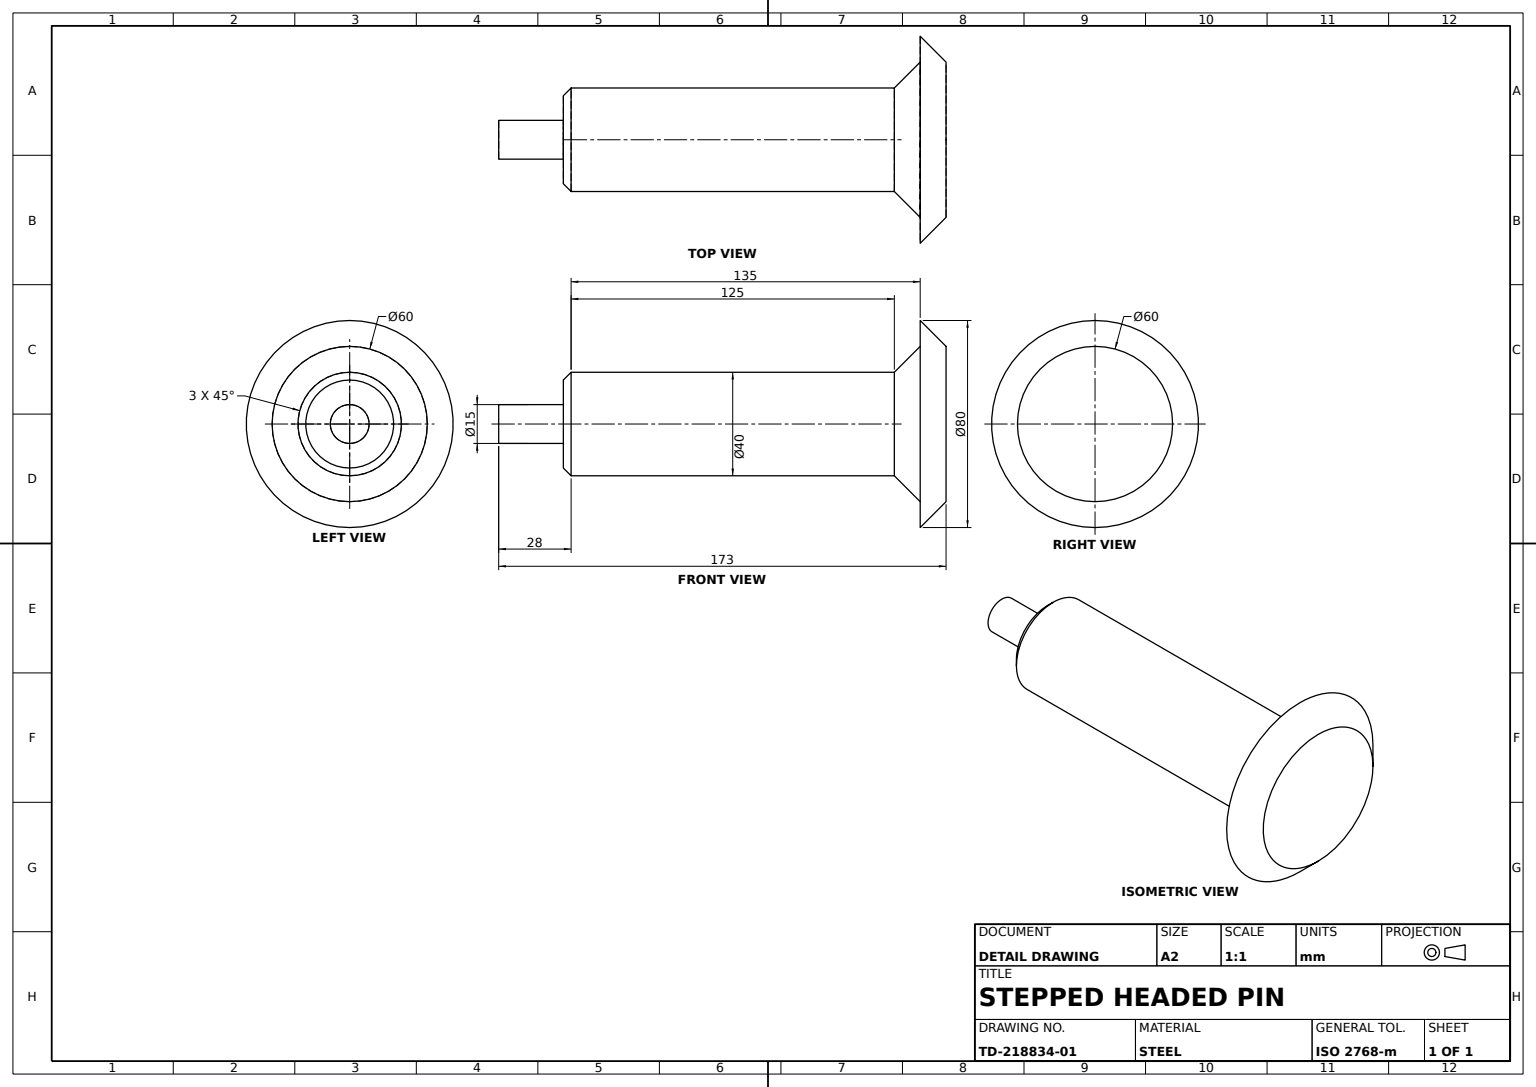
from build123d import *

# Parameters (mm, degrees)
PIN_PROFILE_SKETCH_W   = 25
PIN_PROFILE_SKETCH_H   = 7.5
PIN_PROFILE_SKETCH_W_2 = 125
PIN_PROFILE_SKETCH_H_2 = 20


with BuildPart() as part:
    # Pin Profile Sketch → Pin Body Revolve (revolve)
    with BuildSketch(Plane.XY):
        with Locations((-15.5, 3.75)):
            Rectangle(PIN_PROFILE_SKETCH_W, PIN_PROFILE_SKETCH_H)
        with Locations((62.5, 10)):
            Rectangle(PIN_PROFILE_SKETCH_W_2, PIN_PROFILE_SKETCH_H_2)
        Polygon((-3, 0), (0, 0), (0, 20), (-3, 17), (-3, 7.5), align=None)
        Polygon((125, 0), (135, 0), (135, 30), (125, 20), align=None)
        Polygon((135, 0), (145, 0), (145, 30), (135, 40), (135, 30), align=None)
    revolve(axis=Axis((213.258902513, 0, 0), (-1, 0, 0)))


solid = part.part
